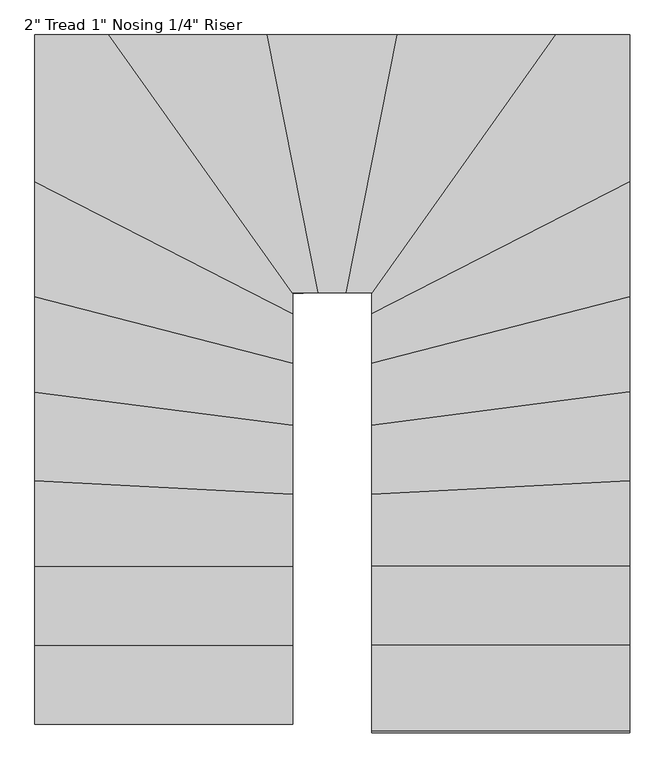
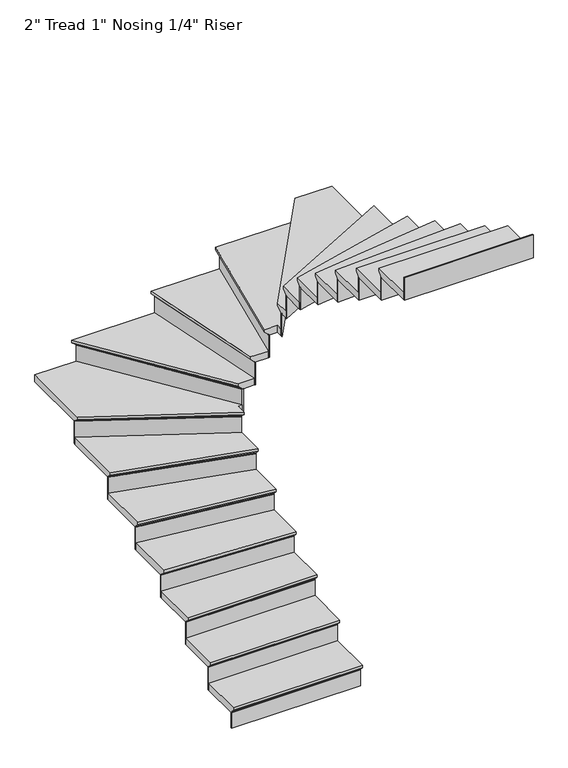
"""IFC4 building model written with IfcOpenShell, lengths in millimetres: stair flight geometry."""

from ifc_helpers import new_model, si_unit, origin, place, context, project, spatial, faceted_brep, source, transform, mapped, element, save


def stair_flight_f188e120(model_context):
    return source(origin(), model_context, "Body", "Brep", [
        faceted_brep([(-12033.8589543, -3829.6838739, 150.2833333), (-12033.8589543, -3829.6838739, 169.3333333), (-12948.2589543, -3829.6838739, 169.3333333), (-12948.2589543, -3829.6838739, 150.2833333), (-12033.8589543, -3804.2838739, 124.8833333), (-12948.2589543, -3804.2838739, 124.8833333), (-12033.8589543, -3524.8838739, 169.3333333), (-12948.2589543, -3524.8838739, 169.3333333), (-12948.2589543, -3804.2838739, 118.5333333), (-12948.2589543, -3524.8838739, 118.5333333), (-12033.8589543, -3524.8838739, 118.5333333), (-12033.8589543, -3804.2838739, 118.5333333)], [[[0, 1, 2, 3]], [[4, 0, 3, 5]], [[2, 1, 6, 7]], [[8, 9, 10, 11]], [[2, 7, 9, 8, 5, 3]], [[8, 11, 4, 5]], [[6, 1, 0, 4, 11, 10]], [[7, 6, 10, 9]]]),
        faceted_brep([(-12033.8589543, -3804.2838739, 118.5333333), (-12033.8589543, -3804.2838739, 0.0), (-12033.8589543, -3797.9338739, 0.0), (-12033.8589543, -3797.9338739, 118.5333333), (-12948.2589543, -3804.2838739, 118.5333333), (-12948.2589543, -3797.9338739, 118.5333333), (-12948.2589543, -3797.9338739, 0.0), (-12948.2589543, -3804.2838739, 0.0)], [[[0, 1, 2, 3]], [[4, 5, 6, 7]], [[1, 0, 4, 7]], [[2, 1, 7, 6]], [[3, 2, 6, 5]], [[0, 3, 5, 4]]]),
        faceted_brep([(-12033.8589543, -3524.8838739, 287.8666667), (-12033.8589543, -3524.8838739, 118.5333333), (-12033.8589543, -3518.5338739, 118.5333333), (-12033.8589543, -3518.5338739, 287.8666667), (-12948.2589543, -3524.8838739, 287.8666667), (-12948.2589543, -3518.5338739, 287.8666667), (-12948.2589543, -3518.5338739, 118.5333333), (-12948.2589543, -3524.8838739, 118.5333333)], [[[0, 1, 2, 3]], [[4, 5, 6, 7]], [[1, 0, 4, 7]], [[2, 1, 7, 6]], [[3, 2, 6, 5]], [[0, 3, 5, 4]]]),
        faceted_brep([(-12948.2589543, -3550.2838739, 338.6666667), (-12033.8589543, -3550.2838739, 338.6666667), (-12033.8589543, -3245.4838739, 338.6666667), (-12948.2589543, -3245.4838739, 338.6666667), (-12948.2589543, -3524.8838739, 287.8666667), (-12948.2589543, -3245.4838739, 287.8666667), (-12033.8589543, -3245.4838739, 287.8666667), (-12033.8589543, -3524.8838739, 287.8666667), (-12948.2589543, -3524.8838739, 294.2166667), (-12948.2589543, -3550.2838739, 319.6166667), (-12033.8589543, -3524.8838739, 294.2166667), (-12033.8589543, -3550.2838739, 319.6166667)], [[[0, 1, 2, 3]], [[4, 5, 6, 7]], [[0, 3, 5, 4, 8, 9]], [[4, 7, 10, 8]], [[2, 1, 11, 10, 7, 6]], [[3, 2, 6, 5]], [[11, 1, 0, 9]], [[10, 11, 9, 8]]]),
        faceted_brep([(-12033.8589543, -3245.4838739, 457.2), (-12033.8589543, -3245.4838739, 287.8666667), (-12033.8589543, -3239.1338739, 287.8666667), (-12033.8589543, -3239.1338739, 457.2), (-12948.2589543, -3245.4838739, 457.2), (-12948.2589543, -3239.1338739, 457.2), (-12948.2589543, -3239.1338739, 287.8666667), (-12948.2589543, -3245.4838739, 287.8666667)], [[[0, 1, 2, 3]], [[4, 5, 6, 7]], [[1, 0, 4, 7]], [[2, 1, 7, 6]], [[3, 2, 6, 5]], [[0, 3, 5, 4]]]),
        faceted_brep([(-12948.2589543, -3270.8838739, 508.0), (-12033.8589543, -3270.8838739, 508.0), (-12033.8589543, -2989.8167124, 508.0), (-12948.2589543, -2942.282442, 508.0), (-12948.2589543, -3245.4838739, 457.2), (-12948.2589543, -2942.282442, 457.2), (-12033.8589543, -2989.8167124, 457.2), (-12033.8589543, -3245.4838739, 457.2), (-12948.2589543, -3245.4838739, 463.55), (-12948.2589543, -3270.8838739, 488.95), (-12033.8589543, -3245.4838739, 463.55), (-12033.8589543, -3270.8838739, 488.95)], [[[0, 1, 2, 3]], [[4, 5, 6, 7]], [[0, 3, 5, 4, 8, 9]], [[4, 7, 10, 8]], [[2, 1, 11, 10, 7, 6]], [[3, 2, 6, 5]], [[11, 1, 0, 9]], [[10, 11, 9, 8]]]),
        faceted_brep([(-12033.8589543, -2989.8167124, 626.5333333), (-12033.8589543, -2989.8167124, 457.2), (-12033.8589543, -2983.4581383, 457.2), (-12033.8589543, -2983.4581383, 626.5333333), (-12948.2589543, -2942.282442, 626.5333333), (-12948.2589543, -2935.9238679, 626.5333333), (-12948.2589543, -2935.9238679, 457.2), (-12948.2589543, -2942.282442, 457.2)], [[[0, 1, 2, 3]], [[4, 5, 6, 7]], [[1, 0, 4, 7]], [[2, 1, 7, 6]], [[3, 2, 6, 5]], [[0, 3, 5, 4]]]),
        faceted_brep([(-12948.2589543, -2967.7167387, 677.3333333), (-12033.8589543, -3015.2510091, 677.3333333), (-12033.8589543, -2745.6500126, 677.3333333), (-12948.2589543, -2627.2939609, 677.3333333), (-12948.2589543, -2942.282442, 626.5333333), (-12948.2589543, -2627.2939609, 626.5333333), (-12033.8589543, -2745.6500126, 626.5333333), (-12033.8589543, -2989.8167124, 626.5333333), (-12948.2589543, -2942.282442, 632.8833333), (-12948.2589543, -2967.7167387, 658.2833333), (-12033.8589543, -2989.8167124, 632.8833333), (-12033.8589543, -3015.2510091, 658.2833333)], [[[0, 1, 2, 3]], [[4, 5, 6, 7]], [[0, 3, 5, 4, 8, 9]], [[4, 7, 10, 8]], [[2, 1, 11, 10, 7, 6]], [[3, 2, 6, 5]], [[11, 1, 0, 9]], [[10, 11, 9, 8]]]),
        faceted_brep([(-12033.8589543, -2745.6500126, 795.8666667), (-12033.8589543, -2745.6500126, 626.5333333), (-12033.8589543, -2739.2470408, 626.5333333), (-12033.8589543, -2739.2470408, 795.8666667), (-12948.2589543, -2627.2939609, 795.8666667), (-12948.2589543, -2620.8909892, 795.8666667), (-12948.2589543, -2620.8909892, 626.5333333), (-12948.2589543, -2627.2939609, 626.5333333)], [[[0, 1, 2, 3]], [[4, 5, 6, 7]], [[1, 0, 4, 7]], [[2, 1, 7, 6]], [[3, 2, 6, 5]], [[0, 3, 5, 4]]]),
        faceted_brep([(-12948.2589543, -2652.9058481, 846.6666667), (-12033.8589543, -2771.2618997, 846.6666667), (-12033.8589543, -2524.0227901, 846.6666667), (-12948.2589543, -2288.8923427, 846.6666667), (-12948.2589543, -2627.2939609, 795.8666667), (-12948.2589543, -2288.8923427, 795.8666667), (-12033.8589543, -2524.0227901, 795.8666667), (-12033.8589543, -2745.6500126, 795.8666667), (-12948.2589543, -2627.2939609, 802.2166667), (-12948.2589543, -2652.9058481, 827.6166667), (-12033.8589543, -2745.6500126, 802.2166667), (-12033.8589543, -2771.2618997, 827.6166667)], [[[0, 1, 2, 3]], [[4, 5, 6, 7]], [[0, 3, 5, 4, 8, 9]], [[4, 7, 10, 8]], [[2, 1, 11, 10, 7, 6]], [[3, 2, 6, 5]], [[11, 1, 0, 9]], [[10, 11, 9, 8]]]),
        faceted_brep([(-12033.8589543, -2524.0227901, 965.2), (-12033.8589543, -2524.0227901, 795.8666667), (-12033.8589543, -2517.4662133, 795.8666667), (-12033.8589543, -2517.4662133, 965.2), (-12948.2589543, -2288.8923427, 965.2), (-12948.2589543, -2282.3357659, 965.2), (-12948.2589543, -2282.3357659, 795.8666667), (-12948.2589543, -2288.8923427, 795.8666667)], [[[0, 1, 2, 3]], [[4, 5, 6, 7]], [[1, 0, 4, 7]], [[2, 1, 7, 6]], [[3, 2, 6, 5]], [[0, 3, 5, 4]]]),
        faceted_brep([(-12948.2589543, -2315.1186502, 1016.0), (-12033.8589543, -2550.2490976, 1016.0), (-12033.8589543, -2347.676154, 1016.0), (-12948.2589543, -1878.8515327, 1016.0), (-12948.2589543, -2288.8923427, 965.2), (-12948.2589543, -1878.8515327, 965.2), (-12033.8589543, -2347.676154, 965.2), (-12033.8589543, -2524.0227901, 965.2), (-12948.2589543, -2288.8923427, 971.55), (-12948.2589543, -2315.1186502, 996.95), (-12033.8589543, -2524.0227901, 971.55), (-12033.8589543, -2550.2490976, 996.95)], [[[0, 1, 2, 3]], [[4, 5, 6, 7]], [[0, 3, 5, 4, 8, 9]], [[4, 7, 10, 8]], [[2, 1, 11, 10, 7, 6]], [[3, 2, 6, 5]], [[11, 1, 0, 9]], [[10, 11, 9, 8]]]),
        faceted_brep([(-12033.8589543, -2347.676154, 1134.5333333), (-12033.8589543, -2347.676154, 965.2), (-12033.8589543, -2340.5401709, 965.2), (-12033.8589543, -2340.5401709, 1134.5333333), (-12948.2589543, -1878.8515327, 1134.5333333), (-12948.2589543, -1871.7155496, 1134.5333333), (-12948.2589543, -1871.7155496, 965.2), (-12948.2589543, -1878.8515327, 965.2)], [[[0, 1, 2, 3]], [[4, 5, 6, 7]], [[1, 0, 4, 7]], [[2, 1, 7, 6]], [[3, 2, 6, 5]], [[0, 3, 5, 4]]]),
        faceted_brep([(-12654.5778206, -1387.552182, 1185.3333333), (-12948.2589543, -1387.552182, 1185.3333333), (-12948.2589543, -1907.3954652, 1185.3333333), (-12033.8589543, -2376.2200866, 1185.3333333), (-12033.8589543, -2301.952182, 1185.3333333), (-12004.3038714, -2301.952182, 1185.3333333), (-12948.2589543, -1387.552182, 1134.5333333), (-12654.5778206, -1387.552182, 1134.5333333), (-12004.3038714, -2301.952182, 1134.5333333), (-12033.8589543, -2301.952182, 1134.5333333), (-12033.8589543, -2347.676154, 1134.5333333), (-12948.2589543, -1878.8515327, 1134.5333333), (-12948.2589543, -1878.8515327, 1140.8833333), (-12948.2589543, -1907.3954652, 1166.2833333), (-12033.8589543, -2347.676154, 1140.8833333), (-12033.8589543, -2376.2200866, 1166.2833333)], [[[0, 1, 2, 3, 4, 5]], [[6, 7, 8, 9, 10, 11]], [[1, 0, 7, 6]], [[2, 1, 6, 11, 12, 13]], [[11, 10, 14, 12]], [[4, 3, 15, 14, 10, 9]], [[5, 4, 9, 8]], [[0, 5, 8, 7]], [[15, 3, 2, 13]], [[14, 15, 13, 12]]]),
        faceted_brep([(-12004.3038714, -2301.952182, 1303.8666667), (-12004.3038714, -2301.952182, 1134.5333333), (-11996.5118966, -2301.952182, 1134.5333333), (-11996.5118966, -2301.952182, 1303.8666667), (-12654.5778206, -1387.552182, 1303.8666667), (-12646.7858458, -1387.552182, 1303.8666667), (-12646.7858458, -1387.552182, 1134.5333333), (-12654.5778206, -1387.552182, 1134.5333333)], [[[0, 1, 2, 3]], [[4, 5, 6, 7]], [[1, 0, 4, 7]], [[2, 1, 7, 6]], [[3, 2, 6, 5]], [[0, 3, 5, 4]]]),
        faceted_brep([(-12685.7457197, -1387.552182, 1354.6666667), (-12035.4717706, -2301.952182, 1354.6666667), (-11917.8497843, -2301.952182, 1354.6666667), (-12098.0906407, -1387.552182, 1354.6666667), (-12654.5778206, -1387.552182, 1303.8666667), (-12098.0906407, -1387.552182, 1303.8666667), (-11917.8497843, -2301.952182, 1303.8666667), (-12004.3038714, -2301.952182, 1303.8666667), (-12654.5778206, -1387.552182, 1310.2166667), (-12685.7457197, -1387.552182, 1335.6166667), (-12004.3038714, -2301.952182, 1310.2166667), (-12035.4717706, -2301.952182, 1335.6166667)], [[[0, 1, 2, 3]], [[4, 5, 6, 7]], [[0, 3, 5, 4, 8, 9]], [[4, 7, 10, 8]], [[2, 1, 11, 10, 7, 6]], [[3, 2, 6, 5]], [[11, 1, 0, 9]], [[10, 11, 9, 8]]]),
        faceted_brep([(-11917.8497843, -2301.952182, 1473.2), (-11917.8497843, -2301.952182, 1303.8666667), (-11911.3775989, -2301.952182, 1303.8666667), (-11911.3775989, -2301.952182, 1473.2), (-12098.0906407, -1387.552182, 1473.2), (-12091.6184552, -1387.552182, 1473.2), (-12091.6184552, -1387.552182, 1303.8666667), (-12098.0906407, -1387.552182, 1303.8666667)], [[[0, 1, 2, 3]], [[4, 5, 6, 7]], [[1, 0, 4, 7]], [[2, 1, 7, 6]], [[3, 2, 6, 5]], [[0, 3, 5, 4]]]),
        faceted_brep([(-12123.9793824, -1387.552182, 1524.0), (-11943.7385261, -2301.952182, 1524.0), (-11818.6906407, -2301.952182, 1524.0), (-11638.4497843, -1387.552182, 1524.0), (-12098.0906407, -1387.552182, 1473.2), (-11638.4497843, -1387.552182, 1473.2), (-11818.6906407, -2301.952182, 1473.2), (-11917.8497843, -2301.952182, 1473.2), (-12098.0906407, -1387.552182, 1479.55), (-12123.9793824, -1387.552182, 1504.95), (-11917.8497843, -2301.952182, 1479.55), (-11943.7385261, -2301.952182, 1504.95)], [[[0, 1, 2, 3]], [[4, 5, 6, 7]], [[0, 3, 5, 4, 8, 9]], [[4, 7, 10, 8]], [[2, 1, 11, 10, 7, 6]], [[3, 2, 6, 5]], [[11, 1, 0, 9]], [[10, 11, 9, 8]]]),
        faceted_brep([(-11818.6906407, -2301.952182, 1642.5333333), (-11818.6906407, -2301.952182, 1473.2), (-11812.2184552, -2301.952182, 1473.2), (-11812.2184552, -2301.952182, 1642.5333333), (-11638.4497843, -1387.552182, 1642.5333333), (-11631.9775989, -1387.552182, 1642.5333333), (-11631.9775989, -1387.552182, 1473.2), (-11638.4497843, -1387.552182, 1473.2)], [[[0, 1, 2, 3]], [[4, 5, 6, 7]], [[1, 0, 4, 7]], [[2, 1, 7, 6]], [[3, 2, 6, 5]], [[0, 3, 5, 4]]]),
        faceted_brep([(-11664.3385261, -1387.552182, 1693.3333333), (-11844.5793824, -2301.952182, 1693.3333333), (-11754.4589543, -2301.952182, 1693.3333333), (-11754.4589543, -2348.0476565, 1693.3333333), (-11071.4042896, -1387.552182, 1693.3333333), (-11638.4497843, -1387.552182, 1642.5333333), (-11071.4042896, -1387.552182, 1642.5333333), (-11754.4589543, -2348.0476565, 1642.5333333), (-11754.4589543, -2301.952182, 1642.5333333), (-11818.6906407, -2301.952182, 1642.5333333), (-11638.4497843, -1387.552182, 1648.8833333), (-11664.3385261, -1387.552182, 1674.2833333), (-11818.6906407, -2301.952182, 1648.8833333), (-11844.5793824, -2301.952182, 1674.2833333)], [[[0, 1, 2, 3, 4]], [[5, 6, 7, 8, 9]], [[0, 4, 6, 5, 10, 11]], [[5, 9, 12, 10]], [[2, 1, 13, 12, 9, 8]], [[3, 2, 8, 7]], [[4, 3, 7, 6]], [[13, 1, 0, 11]], [[12, 13, 11, 10]]]),
        faceted_brep([(-11754.4589543, -2348.0476565, 1811.8666667), (-11754.4589543, -2348.0476565, 1642.5333333), (-11754.4589543, -2359.004549, 1642.5333333), (-11754.4589543, -2359.004549, 1811.8666667), (-11071.4042896, -1387.552182, 1811.8666667), (-11063.6123148, -1387.552182, 1811.8666667), (-11063.6123148, -1387.552182, 1642.5333333), (-11071.4042896, -1387.552182, 1642.5333333)], [[[0, 1, 2, 3]], [[4, 5, 6, 7]], [[1, 0, 4, 7]], [[2, 1, 7, 6]], [[3, 2, 6, 5]], [[0, 3, 5, 4]]]),
        faceted_brep([(-10840.0589543, -1935.9393978, 1862.6666667), (-10840.0589543, -1387.552182, 1862.6666667), (-11102.5721888, -1387.552182, 1862.6666667), (-11754.4589543, -2304.2200866, 1862.6666667), (-11754.4589543, -2404.7640191, 1862.6666667), (-10840.0589543, -1387.552182, 1811.8666667), (-10840.0589543, -1935.9393978, 1811.8666667), (-11754.4589543, -2404.7640191, 1811.8666667), (-11754.4589543, -2348.0476565, 1811.8666667), (-11071.4042896, -1387.552182, 1811.8666667), (-11071.4042896, -1387.552182, 1818.2166667), (-11102.5721888, -1387.552182, 1843.6166667), (-11754.4589543, -2348.0476565, 1818.2166667), (-11754.4589543, -2304.2200866, 1843.6166667)], [[[0, 1, 2, 3, 4]], [[5, 6, 7, 8, 9]], [[1, 0, 6, 5]], [[2, 1, 5, 9, 10, 11]], [[9, 8, 12, 10]], [[4, 3, 13, 12, 8, 7]], [[0, 4, 7, 6]], [[13, 3, 2, 11]], [[12, 13, 11, 10]]]),
        faceted_brep([(-11754.4589543, -2404.7640191, 1981.2), (-11754.4589543, -2404.7640191, 1811.8666667), (-11754.4589543, -2411.9000022, 1811.8666667), (-11754.4589543, -2411.9000022, 1981.2), (-10840.0589543, -1935.9393978, 1981.2), (-10840.0589543, -1943.0753809, 1981.2), (-10840.0589543, -1943.0753809, 1811.8666667), (-10840.0589543, -1935.9393978, 1811.8666667)], [[[0, 1, 2, 3]], [[4, 5, 6, 7]], [[1, 0, 4, 7]], [[2, 1, 7, 6]], [[3, 2, 6, 5]], [[0, 3, 5, 4]]]),
        faceted_brep([(-10840.0589543, -1907.3954652, 2032.0), (-11754.4589543, -2376.2200866, 2032.0), (-11754.4589543, -2576.475405, 2032.0), (-10840.0589543, -2341.3449576, 2032.0), (-10840.0589543, -1935.9393978, 1981.2), (-10840.0589543, -2341.3449576, 1981.2), (-11754.4589543, -2576.475405, 1981.2), (-11754.4589543, -2404.7640191, 1981.2), (-10840.0589543, -1935.9393978, 1987.55), (-10840.0589543, -1907.3954652, 2012.95), (-11754.4589543, -2404.7640191, 1987.55), (-11754.4589543, -2376.2200866, 2012.95)], [[[0, 1, 2, 3]], [[4, 5, 6, 7]], [[0, 3, 5, 4, 8, 9]], [[4, 7, 10, 8]], [[2, 1, 11, 10, 7, 6]], [[3, 2, 6, 5]], [[11, 1, 0, 9]], [[10, 11, 9, 8]]]),
        faceted_brep([(-11754.4589543, -2576.475405, 2150.5333333), (-11754.4589543, -2576.475405, 1981.2), (-11754.4589543, -2583.0319819, 1981.2), (-11754.4589543, -2583.0319819, 2150.5333333), (-10840.0589543, -2341.3449576, 2150.5333333), (-10840.0589543, -2347.9015345, 2150.5333333), (-10840.0589543, -2347.9015345, 1981.2), (-10840.0589543, -2341.3449576, 1981.2)], [[[0, 1, 2, 3]], [[4, 5, 6, 7]], [[1, 0, 4, 7]], [[2, 1, 7, 6]], [[3, 2, 6, 5]], [[0, 3, 5, 4]]]),
        faceted_brep([(-10840.0589543, -2315.1186502, 2201.3333333), (-11754.4589543, -2550.2490976, 2201.3333333), (-11754.4589543, -2796.8737868, 2201.3333333), (-10840.0589543, -2678.5177352, 2201.3333333), (-10840.0589543, -2341.3449576, 2150.5333333), (-10840.0589543, -2678.5177352, 2150.5333333), (-11754.4589543, -2796.8737868, 2150.5333333), (-11754.4589543, -2576.475405, 2150.5333333), (-10840.0589543, -2341.3449576, 2156.8833333), (-10840.0589543, -2315.1186502, 2182.2833333), (-11754.4589543, -2576.475405, 2156.8833333), (-11754.4589543, -2550.2490976, 2182.2833333)], [[[0, 1, 2, 3]], [[4, 5, 6, 7]], [[0, 3, 5, 4, 8, 9]], [[4, 7, 10, 8]], [[2, 1, 11, 10, 7, 6]], [[3, 2, 6, 5]], [[11, 1, 0, 9]], [[10, 11, 9, 8]]]),
        faceted_brep([(-11754.4589543, -2796.8737868, 2319.8666667), (-11754.4589543, -2796.8737868, 2150.5333333), (-11754.4589543, -2803.2767586, 2150.5333333), (-11754.4589543, -2803.2767586, 2319.8666667), (-10840.0589543, -2678.5177352, 2319.8666667), (-10840.0589543, -2684.9207069, 2319.8666667), (-10840.0589543, -2684.9207069, 2150.5333333), (-10840.0589543, -2678.5177352, 2150.5333333)], [[[0, 1, 2, 3]], [[4, 5, 6, 7]], [[1, 0, 4, 7]], [[2, 1, 7, 6]], [[3, 2, 6, 5]], [[0, 3, 5, 4]]]),
        faceted_brep([(-10840.0589543, -2652.9058481, 2370.6666667), (-11754.4589543, -2771.2618997, 2370.6666667), (-11754.4589543, -3040.6853057, 2370.6666667), (-10840.0589543, -2993.1510353, 2370.6666667), (-10840.0589543, -2678.5177352, 2319.8666667), (-10840.0589543, -2993.1510353, 2319.8666667), (-11754.4589543, -3040.6853057, 2319.8666667), (-11754.4589543, -2796.8737868, 2319.8666667), (-10840.0589543, -2678.5177352, 2326.2166667), (-10840.0589543, -2652.9058481, 2351.6166667), (-11754.4589543, -2796.8737868, 2326.2166667), (-11754.4589543, -2771.2618997, 2351.6166667)], [[[0, 1, 2, 3]], [[4, 5, 6, 7]], [[0, 3, 5, 4, 8, 9]], [[4, 7, 10, 8]], [[2, 1, 11, 10, 7, 6]], [[3, 2, 6, 5]], [[11, 1, 0, 9]], [[10, 11, 9, 8]]]),
        faceted_brep([(-11754.4589543, -3040.6853057, 2489.2), (-11754.4589543, -3040.6853057, 2319.8666667), (-11754.4589543, -3047.0438799, 2319.8666667), (-11754.4589543, -3047.0438799, 2489.2), (-10840.0589543, -2993.1510353, 2489.2), (-10840.0589543, -2999.5096095, 2489.2), (-10840.0589543, -2999.5096095, 2319.8666667), (-10840.0589543, -2993.1510353, 2319.8666667)], [[[0, 1, 2, 3]], [[4, 5, 6, 7]], [[1, 0, 4, 7]], [[2, 1, 7, 6]], [[3, 2, 6, 5]], [[0, 3, 5, 4]]]),
        faceted_brep([(-10840.0589543, -2967.7167387, 2540.0), (-11754.4589543, -3015.2510091, 2540.0), (-11754.4589543, -3296.2838739, 2540.0), (-10840.0589543, -3296.2838739, 2540.0), (-10840.0589543, -2993.1510353, 2489.2), (-10840.0589543, -3296.2838739, 2489.2), (-11754.4589543, -3296.2838739, 2489.2), (-11754.4589543, -3040.6853057, 2489.2), (-10840.0589543, -2993.1510353, 2495.55), (-10840.0589543, -2967.7167387, 2520.95), (-11754.4589543, -3040.6853057, 2495.55), (-11754.4589543, -3015.2510091, 2520.95)], [[[0, 1, 2, 3]], [[4, 5, 6, 7]], [[0, 3, 5, 4, 8, 9]], [[4, 7, 10, 8]], [[2, 1, 11, 10, 7, 6]], [[3, 2, 6, 5]], [[11, 1, 0, 9]], [[10, 11, 9, 8]]]),
        faceted_brep([(-11754.4589543, -3296.2838739, 2658.5333333), (-11754.4589543, -3296.2838739, 2489.2), (-11754.4589543, -3302.6338739, 2489.2), (-11754.4589543, -3302.6338739, 2658.5333333), (-10840.0589543, -3296.2838739, 2658.5333333), (-10840.0589543, -3302.6338739, 2658.5333333), (-10840.0589543, -3302.6338739, 2489.2), (-10840.0589543, -3296.2838739, 2489.2)], [[[0, 1, 2, 3]], [[4, 5, 6, 7]], [[1, 0, 4, 7]], [[2, 1, 7, 6]], [[3, 2, 6, 5]], [[0, 3, 5, 4]]]),
        faceted_brep([(-10840.0589543, -3270.8838739, 2709.3333333), (-11754.4589543, -3270.8838739, 2709.3333333), (-11754.4589543, -3575.6838739, 2709.3333333), (-10840.0589543, -3575.6838739, 2709.3333333), (-10840.0589543, -3296.2838739, 2658.5333333), (-10840.0589543, -3575.6838739, 2658.5333333), (-11754.4589543, -3575.6838739, 2658.5333333), (-11754.4589543, -3296.2838739, 2658.5333333), (-10840.0589543, -3296.2838739, 2664.8833333), (-10840.0589543, -3270.8838739, 2690.2833333), (-11754.4589543, -3296.2838739, 2664.8833333), (-11754.4589543, -3270.8838739, 2690.2833333)], [[[0, 1, 2, 3]], [[4, 5, 6, 7]], [[0, 3, 5, 4, 8, 9]], [[4, 7, 10, 8]], [[2, 1, 11, 10, 7, 6]], [[3, 2, 6, 5]], [[11, 1, 0, 9]], [[10, 11, 9, 8]]]),
        faceted_brep([(-11754.4589543, -3575.6838739, 2827.8666667), (-11754.4589543, -3575.6838739, 2658.5333333), (-11754.4589543, -3582.0338739, 2658.5333333), (-11754.4589543, -3582.0338739, 2827.8666667), (-10840.0589543, -3575.6838739, 2827.8666667), (-10840.0589543, -3582.0338739, 2827.8666667), (-10840.0589543, -3582.0338739, 2658.5333333), (-10840.0589543, -3575.6838739, 2658.5333333)], [[[0, 1, 2, 3]], [[4, 5, 6, 7]], [[1, 0, 4, 7]], [[2, 1, 7, 6]], [[3, 2, 6, 5]], [[0, 3, 5, 4]]]),
        faceted_brep([(-11754.4589543, -3855.0838739, 2997.2), (-11754.4589543, -3855.0838739, 2827.8666667), (-11754.4589543, -3861.4338739, 2827.8666667), (-11754.4589543, -3861.4338739, 2997.2), (-10840.0589543, -3855.0838739, 2997.2), (-10840.0589543, -3861.4338739, 2997.2), (-10840.0589543, -3861.4338739, 2827.8666667), (-10840.0589543, -3855.0838739, 2827.8666667)], [[[0, 1, 2, 3]], [[4, 5, 6, 7]], [[1, 0, 4, 7]], [[2, 1, 7, 6]], [[3, 2, 6, 5]], [[0, 3, 5, 4]]]),
        faceted_brep([(-10840.0589543, -3550.2838739, 2878.6666667), (-11754.4589543, -3550.2838739, 2878.6666667), (-11754.4589543, -3855.0838739, 2878.6666667), (-10840.0589543, -3855.0838739, 2878.6666667), (-10840.0589543, -3575.6838739, 2827.8666667), (-10840.0589543, -3855.0838739, 2827.8666667), (-11754.4589543, -3855.0838739, 2827.8666667), (-11754.4589543, -3575.6838739, 2827.8666667), (-10840.0589543, -3575.6838739, 2834.2166667), (-10840.0589543, -3550.2838739, 2859.6166667), (-11754.4589543, -3575.6838739, 2834.2166667), (-11754.4589543, -3550.2838739, 2859.6166667)], [[[0, 1, 2, 3]], [[4, 5, 6, 7]], [[0, 3, 5, 4, 8, 9]], [[4, 7, 10, 8]], [[2, 1, 11, 10, 7, 6]], [[3, 2, 6, 5]], [[11, 1, 0, 9]], [[10, 11, 9, 8]]]),
    ])


if __name__ == "__main__":
    model = new_model("IFC4")
    model_context = context("Model", 3, world=origin())
    ifc_project = project(units=[si_unit("LENGTHUNIT", "METRE", prefix="MILLI")], contexts=[model_context])
    site = spatial("IfcSite", under=ifc_project)
    building = spatial("IfcBuilding", under=site)
    placement = place(None, origin())
    stair_flight_shape = stair_flight_f188e120(model_context)
    element("IfcStairFlight", 1, ObjectType="2\" Tread 1\" Nosing 1/4\" Riser", at=placement, inside=building, context=model_context, shape_type="MappedRepresentation", body=[
        mapped(stair_flight_shape, transform((0.0, 0.0, 0.0), x_axis=(1.0, 0.0, 0.0), y_axis=(0.0, 1.0, 0.0), z_axis=(0.0, 0.0, 1.0))),
    ])
    save(model, "model.ifc")
